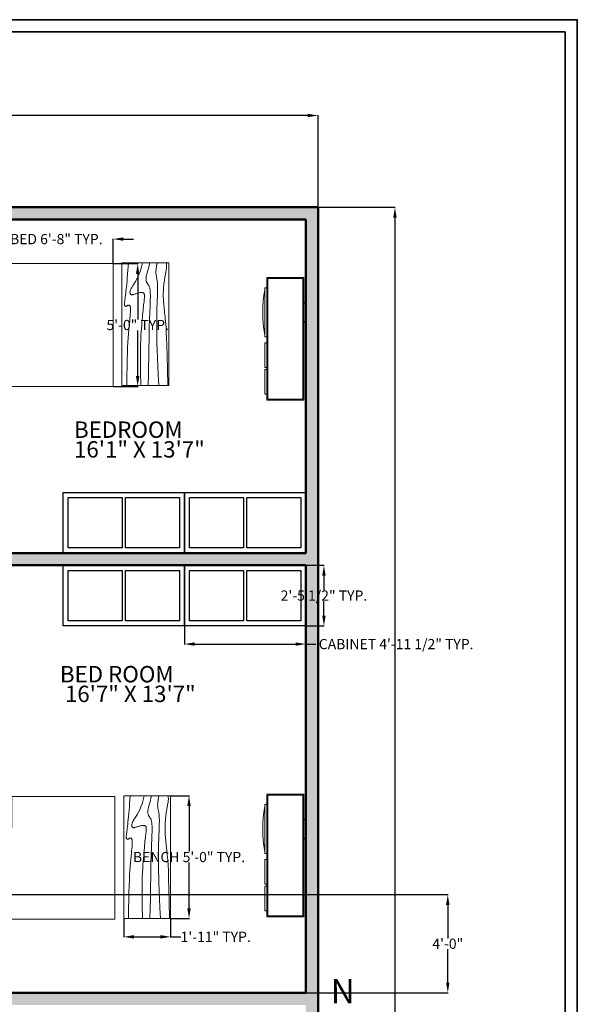
# Model space of a CAD drawing. Units: inches. Extents: x -60 to 743, y -483 to 510.
# Tile 7 of 7: x 470 to 743, y 29 to 510. Entities that reach past the tile are written whole.
import ezdxf

# ---------------------------------------------------------------- set-up
doc = ezdxf.new("R2010")
doc.units = ezdxf.units.IN
doc.header["$MEASUREMENT"] = 0
for name, color, linetype, lineweight in [('A-ANNO-DIMS', 2, 'Continuous', 18), ('A-ANNO-SYMB', 7, 'Continuous', 18), ('A-ANNO-TTLB', 7, 'Continuous', 35), ('A-AREA-IDEN', 7, 'Continuous', 25), ('A-FLOR-CASE', 40, 'Continuous', 25), ('A-WALL-PATT', 30, 'Continuous', 13), ('FURNITURE', 40, 'Continuous', 18), ('WALL BOUNDRY', 10, 'Continuous', 50)]:
    doc.layers.add(name, color=color, linetype=linetype, lineweight=lineweight)
doc.styles.get("Standard").update_dxf_attribs({"font": 'arial.ttf'})
doc.dimstyles.get("Standard").update_dxf_attribs({"dimtxt": 5, "dimasz": 5, "dimexe": 0.18, "dimexo": 0.0625, "dimgap": 0.09, "dimtad": 0, "dimtih": 1, "dimtoh": 1, "dimdec": 1, "dimzin": 0, "dimdsep": 46, "dimlunit": 4, "dimtxsty": 'Standard', "dimcen": 0.09, "dimadec": 0, "dimazin": 0, "dimtfac": 1, "dimtdec": 1, "dimtofl": 0, "dimtmove": 0, "dimatfit": 3, "dimfxl": 1, "dimtolj": 1, "dimtzin": 0, "dimarcsym": 0})

# ---------------------------------------------------------------- blocks, each defined once
blk = doc.blocks.new('Wall Cabinet - 18 x 36 in front')
for p, q in [((17.5, -1.5), (17.5, -16.5)), ((18.5, -16.5), (18.5, -1.5))]:
    blk.add_line(p, q)
blk.add_lwpolyline([(0, -18), (0, 0), (36, 0), (36, -18)], close=True)
for points in [[(17.5, -16.5), (1.5, -16.5), (1.5, -1.5), (17.5, -1.5)], [(18.5, -1.5), (34.5, -1.5), (34.5, -16.5), (18.5, -16.5)]]:
    blk.add_lwpolyline(points)
blk = doc.blocks.new('Bed - Queen')
for p, q in [((0, -80.00003), (0, 0)), ((0, 0), (59.99999, 0)), ((59.99999, 0), (59.99999, -80.00003)), ((7.99999, -1.2), (28.79998, -1.2)), ((7.99999, -14.4), (7.99999, -1.2)), ((28.79998, -1.2), (28.79998, -14.4)), ((31.19999, -1.2), (51.99999, -1.2)), ((31.19999, -14.4), (31.19999, -1.2)), ((51.99999, -1.2), (51.99999, -16.4)), ((0, -14.4), (44.8, -14.4)), ((59.99999, -29.6), (44.8, -14.4)), ((44.8, -14.4), (44.8, -29.6)), ((44.8, -16.8), (0, -16.8)), ((51.99999, -16.4), (46.79936, -16.4)), ((44.8, -29.6), (59.99999, -29.6)), ((59.99999, -80.00003), (0, -80.00003))]:
    blk.add_line(p, q)
blk = doc.blocks.new('Entertainment Center')
for p, q in [((-4, 0), (-5, -1)), ((4, 0), (-4, 0)), ((5, -1), (4, 0)), ((-17, -19), (-17, -1)), ((-17, -1), (43, -1)), ((-16.5, -18.5), (-16.5, -1.5)), ((-16.5, -1.5), (42.5, -1.5)), ((42.5, -1.5), (42.5, -18.5)), ((43, -1), (43, -19)), ((43, -19), (-17, -19)), ((42.5, -18.5), (-16.5, -18.5)), ((-12, -20), (-12, -19)), ((12, -19), (12, -20)), ((15, -20), (15, -19)), ((27, -19), (27, -20)), ((28, -20), (28, -19)), ((40, -19), (40, -20)), ((12, -20), (-12, -20)), ((27, -20), (15, -20)), ((40, -20), (28, -20))]:
    blk.add_line(p, q)
blk.add_arc((0, 40), 61, 259.6111, 280.3889)
blk = doc.blocks.new('*D22')
at = {"layer": 'A-ANNO-DIMS', "color": 0, "lineweight": -2, "transparency": 16777216}
for p, q in [((13.15, 418.48), (13.15, 463.48)), ((18.15, 463.3), (310.31, 463.3)), ((611.15, 463.3), (318.98, 463.3)), ((616.15, 418.48), (616.15, 463.48))]:
    blk.add_line(p, q, dxfattribs=at)
at = {"layer": 'A-ANNO-DIMS', "color": 0, "transparency": 16777216}
for points in [[(18.15, 464.13), (18.15, 462.46), (13.15, 463.3)], [(611.15, 464.13), (611.15, 462.46), (616.15, 463.3)]]:
    blk.add_solid(points, dxfattribs=at)
at = {"layer": 'Defpoints', "color": 0, "transparency": 16777216}
for p in [(616.15, 463.3), (13.15, 418.42), (616.15, 418.42)]:
    blk.add_point(p, dxfattribs=at)
at = {"layer": 'A-ANNO-DIMS', "color": 0, "transparency": 16777216, "insert": (314.65, 463.3), "char_height": 5, "attachment_point": 5}
blk.add_mtext("\\A1;50'", dxfattribs=at)
blk = doc.blocks.new('*D23')
at = {"layer": 'A-ANNO-DIMS', "color": 0, "lineweight": -2, "transparency": 16777216}
for p, q in [((616.21, 418.42), (653.91, 418.42)), ((653.73, 413.42), (653.73, 1.06)), ((653.73, -416.58), (653.73, -4.22)), ((616.21, -421.58), (653.91, -421.58))]:
    blk.add_line(p, q, dxfattribs=at)
at = {"layer": 'A-ANNO-DIMS', "color": 0, "transparency": 16777216}
for points in [[(652.9, 413.42), (654.56, 413.42), (653.73, 418.42)], [(652.9, -416.58), (654.56, -416.58), (653.73, -421.58)]]:
    blk.add_solid(points, dxfattribs=at)
at = {"layer": 'Defpoints', "color": 0, "transparency": 16777216}
for p in [(616.15, 418.42), (616.15, -421.58), (653.73, -421.58)]:
    blk.add_point(p, dxfattribs=at)
at = {"layer": 'A-ANNO-DIMS', "color": 0, "transparency": 16777216, "insert": (653.73, -1.58), "char_height": 5, "attachment_point": 5}
blk.add_mtext("\\A1;70'", dxfattribs=at)
blk = doc.blocks.new('BENCH-WOOD-60IN')
blk.add_lwpolyline([(22.9143, 0), (22.9143, 60), (0, 60), (0, 0)], close=True)
for points in [[(2.4, 0), (2.418, 4.8155), (2.4688, 9.0302), (2.5477, 12.709), (2.65, 15.9167), (2.7711, 18.7181), (2.9063, 21.1781), (3.0508, 23.3616), (3.2, 25.3333), (3.3495, 27.1477), (3.4958, 28.8172), (3.636, 30.3437), (3.7667, 31.7291), (3.8849, 32.9756), (3.9875, 34.0849), (4.0714, 35.059), (4.1334, 35.9), (4.1711, 36.6114), (4.1854, 37.2041), (4.1779, 37.6906), (4.15, 38.0833), (4.1034, 38.3948), (4.0396, 38.6375), (3.9602, 38.8239), (3.8667, 38.9666), (3.7608, 39.0764), (3.6448, 39.1573), (3.521, 39.2116), (3.3917, 39.2416), (3.2593, 39.2498), (3.1261, 39.2385), (2.9944, 39.21), (2.8667, 39.1666), (2.7447, 39.111), (2.6281, 39.0468), (2.5163, 38.978), (2.4083, 38.9083), (2.3035, 38.8418), (2.201, 38.7823), (2.1001, 38.7337), (2, 38.7), (1.9003, 38.6844), (1.8021, 38.6875), (1.707, 38.7094), (1.6167, 38.75), (1.5326, 38.8094), (1.4563, 38.8875), (1.3893, 38.9844), (1.3333, 39.1), (1.2896, 39.2351), (1.2583, 39.3937), (1.2396, 39.5804), (1.2333, 39.8), (1.2396, 40.057), (1.2583, 40.3562), (1.2896, 40.7023), (1.3333, 41.1), (1.3895, 41.5547), (1.4573, 42.0755), (1.5361, 42.6721), (1.625, 43.3542), (1.7233, 44.1316), (1.8302, 45.014), (1.9449, 46.0114), (2.0667, 47.1333), (2.1947, 48.3862), (2.3281, 49.7625), (2.4663, 51.2513), (2.6083, 52.8416), (2.7535, 54.5226), (2.9011, 56.2833), (3.0501, 58.1127), (3.2, 60)], [(9.2, 0), (9.0858, 6.5759), (9.0365, 11.9385), (9.0418, 16.2527), (9.0917, 19.6833), (9.1759, 22.3952), (9.2844, 24.5531), (9.4069, 26.322), (9.5333, 27.8666), (9.6553, 29.3241), (9.7719, 30.7203), (9.8837, 32.0532), (9.9917, 33.3208), (10.0965, 34.5213), (10.199, 35.6526), (10.2999, 36.7128), (10.4, 37.7), (10.4996, 38.6129), (10.5969, 39.4531), (10.6895, 40.223), (10.775, 40.925), (10.8512, 41.5613), (10.9156, 42.1344), (10.966, 42.6465), (11, 43.1), (11.0158, 43.4976), (11.0136, 43.8437), (10.9942, 44.143), (10.9583, 44.4), (10.9069, 44.6195), (10.8406, 44.8062), (10.7603, 44.9648), (10.6667, 45.1), (10.5598, 45.2155), (10.4365, 45.3114), (10.2929, 45.3871), (10.125, 45.4416), (9.929, 45.4743), (9.7011, 45.4844), (9.4371, 45.4709), (9.1333, 45.4333), (8.7883, 45.3716), (8.4104, 45.2896), (8.0107, 45.1919), (7.6, 45.0833), (7.1893, 44.9685), (6.7896, 44.8521), (6.4117, 44.7388), (6.0667, 44.6333), (5.7628, 44.54), (5.4979, 44.4614), (5.2675, 44.4001), (5.0667, 44.3583), (4.8909, 44.3384), (4.7354, 44.3427), (4.5956, 44.3736), (4.4667, 44.4333), (4.3453, 44.5236), (4.2333, 44.6427), (4.1339, 44.7884), (4.05, 44.9583), (3.9849, 45.1501), (3.9417, 45.3614), (3.9234, 45.59), (3.9333, 45.8333), (3.9749, 46.0915), (4.0531, 46.3734), (4.1736, 46.6906), (4.3417, 47.0542), (4.5629, 47.4756), (4.8427, 47.9661), (5.1866, 48.5372), (5.6, 49.2), (6.0844, 49.9676), (6.625, 50.8594), (7.2031, 51.8965), (7.8, 53.1), (8.3969, 54.491), (8.975, 56.0906), (9.5156, 57.9199), (10, 60)], [(12.8, 0), (12.9322, 5.1847), (13.0323, 9.6213), (13.1059, 13.3963), (13.1583, 16.5958), (13.1952, 19.3063), (13.2219, 21.614), (13.2439, 23.6054), (13.2667, 25.3666), (13.2947, 26.9728), (13.3281, 28.4531), (13.3663, 29.8256), (13.4083, 31.1083), (13.4535, 32.3191), (13.501, 33.476), (13.5501, 34.597), (13.6, 35.7), (13.6497, 36.7984), (13.6979, 37.8875), (13.743, 38.9578), (13.7833, 40), (13.8174, 41.0047), (13.8438, 41.9625), (13.8607, 42.864), (13.8667, 43.7), (13.8604, 44.4631), (13.8417, 45.1552), (13.8104, 45.7801), (13.7667, 46.3416), (13.7104, 46.8439), (13.6417, 47.2906), (13.5604, 47.6858), (13.4667, 48.0333), (13.3608, 48.3375), (13.2448, 48.6042), (13.121, 48.8396), (12.9917, 49.05), (12.8593, 49.2417), (12.7261, 49.4208), (12.5944, 49.5937), (12.4667, 49.7667), (12.3451, 49.9452), (12.2313, 50.1323), (12.1268, 50.3303), (12.0333, 50.5416), (11.9524, 50.7686), (11.8854, 51.0135), (11.8341, 51.2788), (11.8, 51.5666), (11.7843, 51.8785), (11.7865, 52.2116), (11.8059, 52.562), (11.8417, 52.926), (11.8931, 53.2998), (11.9594, 53.6795), (12.0397, 54.0614), (12.1333, 54.4416), (12.2401, 54.8223), (12.3625, 55.2293), (12.5037, 55.6942), (12.6667, 56.2489), (12.8547, 56.9251), (13.0708, 57.7545), (13.3182, 58.7689), (13.6, 60)], [(18, 0), (17.7273, 5.124), (17.5057, 9.6609), (17.3303, 13.6705), (17.1958, 17.2125), (17.0973, 20.3467), (17.0297, 23.1328), (16.9878, 25.6307), (16.9667, 27.9), (16.9617, 29.9928), (16.9703, 31.9302), (16.9907, 33.7254), (17.0208, 35.3917), (17.0588, 36.9423), (17.1026, 38.3906), (17.1503, 39.7499), (17.2, 41.0333), (17.2496, 42.2519), (17.2969, 43.4073), (17.3395, 44.4986), (17.375, 45.525), (17.4012, 46.4858), (17.4156, 47.3802), (17.416, 48.2074), (17.4, 48.9667), (17.3662, 49.6583), (17.3167, 50.2872), (17.2547, 50.8595), (17.1833, 51.3812), (17.1057, 51.8584), (17.025, 52.2971), (16.9443, 52.7034), (16.8667, 53.0833), (16.7951, 53.443), (16.7313, 53.789), (16.6768, 54.128), (16.6334, 54.4666), (16.6024, 54.8115), (16.5854, 55.1693), (16.5841, 55.5465), (16.6, 55.95), (16.6337, 56.3828), (16.6823, 56.8346), (16.7418, 57.2915), (16.8084, 57.7396), (16.878, 58.165), (16.9469, 58.5539), (17.0111, 58.8924), (17.0667, 59.1666), (17.1107, 59.3679), (17.1438, 59.5078), (17.1675, 59.6032), (17.1833, 59.6708), (17.193, 59.7275), (17.1979, 59.7901), (17.1998, 59.8753), (17.2, 60)], [(22.4, 0), (22.2501, 8.0098), (22.1011, 14.4094), (21.9535, 19.4168), (21.8083, 23.25), (21.6663, 26.1269), (21.5281, 28.2656), (21.3947, 29.884), (21.2667, 31.2), (21.1448, 32.3967), (21.0292, 33.5172), (20.9198, 34.5697), (20.8167, 35.5625), (20.7198, 36.5037), (20.6292, 37.4015), (20.5448, 38.2642), (20.4667, 39.1), (20.3951, 39.9164), (20.3313, 40.7187), (20.2768, 41.5117), (20.2333, 42.3), (20.2024, 43.0883), (20.1854, 43.8812), (20.1841, 44.6836), (20.2, 45.5), (20.234, 46.3328), (20.2844, 47.1747), (20.3488, 48.0163), (20.425, 48.8479), (20.5106, 49.66), (20.6031, 50.4429), (20.7004, 51.1872), (20.8, 51.8833), (20.8999, 52.5246), (20.9995, 53.1166), (21.0983, 53.6681), (21.1958, 54.1875), (21.2919, 54.6834), (21.3859, 55.1646), (21.4777, 55.6394), (21.5667, 56.1167), (21.6515, 56.6028), (21.7266, 57.0961), (21.7852, 57.5929), (21.8208, 58.0896), (21.8268, 58.5823), (21.7964, 59.0674), (21.723, 59.5412), (21.6, 60)]]:
    blk.add_lwpolyline(points)
blk = doc.blocks.new('*D30')
at = {"layer": 'A-ANNO-DIMS', "color": 0, "lineweight": -2, "transparency": 16777216}
for p, q in [((550.88, 213.73), (550.88, 204.72)), ((610.15, 213.73), (610.15, 204.72)), ((555.88, 204.9), (605.15, 204.9)), ((610.15, 204.9), (615.15, 204.9))]:
    blk.add_line(p, q, dxfattribs=at)
at = {"layer": 'A-ANNO-DIMS', "color": 0, "transparency": 16777216}
for points in [[(555.88, 205.73), (555.88, 204.07), (550.88, 204.9)], [(605.15, 205.73), (605.15, 204.07), (610.15, 204.9)]]:
    blk.add_solid(points, dxfattribs=at)
at = {"layer": 'Defpoints', "color": 0, "transparency": 16777216}
for p in [(550.88, 213.79), (610.15, 213.79), (610.15, 204.9)]:
    blk.add_point(p, dxfattribs=at)
at = {"layer": 'A-ANNO-DIMS', "color": 0, "transparency": 16777216, "insert": (654.32, 204.9), "char_height": 5, "attachment_point": 5}
blk.add_mtext('\\A1;CABINET 4\'-11 1/2" TYP.', dxfattribs=at)
blk = doc.blocks.new('*D31')
at = {"layer": 'A-ANNO-DIMS', "color": 0, "lineweight": -2, "transparency": 16777216}
for p, q in [((610.21, 243.42), (619.22, 243.42)), ((619.04, 238.42), (619.04, 231.28)), ((619.04, 218.79), (619.04, 225.93)), ((610.21, 213.79), (619.22, 213.79))]:
    blk.add_line(p, q, dxfattribs=at)
at = {"layer": 'A-ANNO-DIMS', "color": 0, "transparency": 16777216}
for points in [[(618.2, 238.42), (619.87, 238.42), (619.04, 243.42)], [(618.2, 218.79), (619.87, 218.79), (619.04, 213.79)]]:
    blk.add_solid(points, dxfattribs=at)
at = {"layer": 'Defpoints', "color": 0, "transparency": 16777216}
for p in [(610.15, 243.42), (619.04, 243.42), (610.15, 213.79)]:
    blk.add_point(p, dxfattribs=at)
at = {"layer": 'A-ANNO-DIMS', "color": 0, "transparency": 16777216, "insert": (619.04, 228.61), "char_height": 5, "attachment_point": 5}
blk.add_mtext('\\A1;2\'-5 1/2" TYP.', dxfattribs=at)
blk = doc.blocks.new('*D50')
at = {"layer": 'A-ANNO-DIMS', "color": 0, "lineweight": -2, "transparency": 16777216}
for p, q in [((431.03, 402.88), (426.03, 402.88)), ((436.03, 390.95), (436.03, 403.06)), ((516.03, 390.95), (516.03, 403.06)), ((521.03, 402.88), (526.03, 402.88))]:
    blk.add_line(p, q, dxfattribs=at)
at = {"layer": 'A-ANNO-DIMS', "color": 0, "transparency": 16777216}
for points in [[(431.03, 403.72), (431.03, 402.05), (436.03, 402.88)], [(521.03, 403.72), (521.03, 402.05), (516.03, 402.88)]]:
    blk.add_solid(points, dxfattribs=at)
at = {"layer": 'Defpoints', "color": 0, "transparency": 16777216}
for p in [(436.03, 402.88), (436.03, 390.88), (516.03, 390.88)]:
    blk.add_point(p, dxfattribs=at)
at = {"layer": 'A-ANNO-DIMS', "color": 0, "transparency": 16777216, "insert": (476.03, 402.88), "char_height": 5, "attachment_point": 5}
blk.add_mtext('\\A1;QUEEN BED 6\'-8" TYP.', dxfattribs=at)
blk = doc.blocks.new('*D51')
at = {"layer": 'A-ANNO-DIMS', "color": 0, "lineweight": -2, "transparency": 16777216}
for p, q in [((516.09, 390.88), (528.21, 390.88)), ((528.03, 385.88), (528.03, 363.53)), ((528.03, 335.88), (528.03, 358.24)), ((516.09, 330.88), (528.21, 330.88))]:
    blk.add_line(p, q, dxfattribs=at)
at = {"layer": 'A-ANNO-DIMS', "color": 0, "transparency": 16777216}
for points in [[(527.19, 385.88), (528.86, 385.88), (528.03, 390.88)], [(527.19, 335.88), (528.86, 335.88), (528.03, 330.88)]]:
    blk.add_solid(points, dxfattribs=at)
at = {"layer": 'Defpoints', "color": 0, "transparency": 16777216}
for p in [(516.03, 390.88), (528.03, 390.88), (516.03, 330.88)]:
    blk.add_point(p, dxfattribs=at)
at = {"layer": 'A-ANNO-DIMS', "color": 0, "transparency": 16777216, "insert": (528.03, 360.88), "char_height": 5, "attachment_point": 5}
blk.add_mtext('\\A1;5\'-0" TYP.', dxfattribs=at)
blk = doc.blocks.new('*D52')
at = {"layer": 'A-ANNO-DIMS', "color": 0, "lineweight": -2, "transparency": 16777216}
for p, q in [((544.18, 130.8), (553.29, 130.8)), ((553.11, 125.8), (553.11, 103.47)), ((553.11, 75.8), (553.11, 98.12)), ((544.18, 70.8), (553.29, 70.8))]:
    blk.add_line(p, q, dxfattribs=at)
at = {"layer": 'A-ANNO-DIMS', "color": 0, "transparency": 16777216}
for points in [[(552.28, 125.8), (553.95, 125.8), (553.11, 130.8)], [(552.28, 75.8), (553.95, 75.8), (553.11, 70.8)]]:
    blk.add_solid(points, dxfattribs=at)
at = {"layer": 'Defpoints', "color": 0, "transparency": 16777216}
for p in [(544.11, 130.8), (553.11, 130.8), (544.11, 70.8)]:
    blk.add_point(p, dxfattribs=at)
at = {"layer": 'A-ANNO-DIMS', "color": 0, "transparency": 16777216, "insert": (553.11, 100.8), "char_height": 5, "attachment_point": 5}
blk.add_mtext('\\A1;BENCH 5\'-0" TYP.', dxfattribs=at)
blk = doc.blocks.new('*D53')
at = {"layer": 'A-ANNO-DIMS', "color": 0, "lineweight": -2, "transparency": 16777216}
for p, q in [((521.2, 70.74), (521.2, 61.62)), ((544.11, 70.74), (544.11, 61.62)), ((526.2, 61.8), (539.11, 61.8)), ((544.11, 61.8), (549.11, 61.8))]:
    blk.add_line(p, q, dxfattribs=at)
at = {"layer": 'A-ANNO-DIMS', "color": 0, "transparency": 16777216}
for points in [[(526.2, 62.63), (526.2, 60.97), (521.2, 61.8)], [(539.11, 62.63), (539.11, 60.97), (544.11, 61.8)]]:
    blk.add_solid(points, dxfattribs=at)
at = {"layer": 'Defpoints', "color": 0, "transparency": 16777216}
for p in [(521.2, 70.8), (544.11, 70.8), (544.11, 61.8)]:
    blk.add_point(p, dxfattribs=at)
at = {"layer": 'A-ANNO-DIMS', "color": 0, "transparency": 16777216, "insert": (566.15, 61.8), "char_height": 5, "attachment_point": 5}
blk.add_mtext('\\A1;1\'-11" TYP.', dxfattribs=at)
blk = doc.blocks.new('*D74')
at = {"layer": 'A-ANNO-DIMS', "color": 0, "lineweight": -2, "transparency": 16777216}
for p, q in [((187.21, 82.42), (679.73, 82.42)), ((679.55, 77.42), (679.55, 61.06)), ((679.55, 39.42), (679.55, 55.78)), ((187.21, 34.42), (679.73, 34.42))]:
    blk.add_line(p, q, dxfattribs=at)
at = {"layer": 'A-ANNO-DIMS', "color": 0, "transparency": 16777216}
for points in [[(678.72, 77.42), (680.39, 77.42), (679.55, 82.42)], [(678.72, 39.42), (680.39, 39.42), (679.55, 34.42)]]:
    blk.add_solid(points, dxfattribs=at)
at = {"layer": 'Defpoints', "color": 0, "transparency": 16777216}
for p in [(187.15, 82.42), (679.55, 82.42), (187.15, 34.42)]:
    blk.add_point(p, dxfattribs=at)
at = {"layer": 'A-ANNO-DIMS', "color": 0, "transparency": 16777216, "insert": (679.55, 58.42), "char_height": 5, "attachment_point": 5}
blk.add_mtext('\\A1;4\'-0"', dxfattribs=at)

msp = doc.modelspace()

# ---------------------------------------------------------------- hatches: boundary and pattern name
at = {"layer": 'A-WALL-PATT'}
h = msp.add_hatch(color=256, dxfattribs=at)
h.dxf.hatch_style = 1
h.paths.add_polyline_path([(412.35, 168.77), (415.89, 168.77), (415.89, 114.92), (412.35, 114.92)], flags=16)
h.paths.add_polyline_path([(87.81, -138.81), (87.81, -142.35), (48.31, -142.32), (48.31, -138.78)], flags=16)
h.paths.add_polyline_path([(459.53, -138.78), (513.39, -138.78), (513.39, -142.32), (459.53, -142.32)], flags=16)
h.paths.add_polyline_path([(164.84, -257.78), (218.7, -257.78), (218.7, -261.32), (164.84, -261.32)], flags=16)
h.paths.add_polyline_path([(417.15, 114.92), (415.89, 114.92), (415.89, 168.77), (417.15, 168.77), (417.15, 195.42), (411.15, 195.42), (411.15, 168.77), (412.35, 168.77), (412.35, 114.92), (411.15, 114.92), (411.15, 28.42), (610.15, 28.42), (610.15, -43.58), (508.15, -43.58), (508.15, -49.58), (610.15, -49.58), (610.15, -137.58), (513.39, -137.58), (513.39, -138.78), (459.53, -138.78), (459.53, -137.58), (359.15, -137.58), (359.15, -143.58), (377.15, -143.58), (377.15, -292.58), (383.15, -292.58), (383.15, -143.58), (459.53, -143.58), (459.53, -142.32), (513.39, -142.32), (513.39, -143.58), (610.15, -143.58), (610.15, -415.58), (610.15, -421.58), (616.15, -421.58), (616.15, 418.42), (13.15, 418.42), (13.15, -421.58), (19.15, -421.58), (430.15, -421.58), (430.15, -415.58), (19.15, -415.58), (19.15, -143.58), (48.31, -143.58), (48.31, -142.32), (87.81, -142.35), (87.81, -143.58), (117.15, -143.58), (117.15, -262.58), (164.84, -262.58), (164.84, -261.32), (218.7, -261.32), (218.7, -262.58), (273.15, -262.58), (273.15, -292.58), (279.15, -292.58), (279.15, -143.58), (297.15, -143.58), (297.15, -137.58), (273.15, -137.58), (273.15, -256.58), (218.7, -256.58), (218.7, -257.78), (164.84, -257.78), (164.84, -256.58), (123.15, -256.58), (123.15, -143.58), (225.15, -143.58), (225.15, -137.58), (87.81, -137.58), (87.81, -138.81), (48.31, -138.78), (48.31, -137.58), (19.15, -137.58), (19.15, 28.42), (187.15, 28.42), (187.15, 34.42), (19.15, 34.42), (19.15, 178.42), (273.15, 178.42), (273.15, 184.42), (19.15, 184.42), (19.15, 345.58), (195.14, 345.58), (195.14, 348.9), (19.15, 348.9), (19.15, 412.42), (267.15, 412.42), (267.15, 319.83), (273.15, 319.83), (273.15, 412.42), (411.15, 412.42), (411.15, 376.24), (417.15, 376.24), (417.15, 412.42), (610.15, 412.42), (610.15, 249.42), (411.15, 249.42), (411.15, 243.42), (610.15, 243.42), (610.15, 34.42), (417.15, 34.42)])

# ---------------------------------------------------------------- linework, layer by layer
at = {"layer": 'A-ANNO-TTLB'}
for points in [[(742.84, -483.31), (-60.19, -483.31), (-60.19, 510.12), (742.84, 510.12)], [(736.84, -477.31), (-54.19, -477.31), (-54.19, 504.12), (736.84, 504.12)]]:
    msp.add_lwpolyline(points, close=True, dxfattribs=at)
at = {"layer": 'WALL BOUNDRY'}
msp.add_lwpolyline([(610.15, -415.58), (610.15, -421.58), (616.15, -421.58), (616.15, 418.42), (13.15, 418.42), (13.15, -421.58), (19.15, -421.58), (430.15, -421.58), (430.15, -415.58), (19.15, -415.58), (19.15, -143.58), (117.15, -143.58), (117.15, -262.58), (273.15, -262.58), (273.15, -292.58), (279.15, -292.58), (377.15, -292.58), (383.15, -292.58), (383.15, -143.58), (610.15, -143.58)], close=True, dxfattribs=at)
for points in [[(417.15, 412.42), (610.15, 412.42), (610.15, 249.42), (411.15, 249.42)], [(411.15, 243.42), (610.15, 243.42), (610.15, 34.42), (417.15, 34.42)]]:
    msp.add_lwpolyline(points, dxfattribs=at)

# ---------------------------------------------------------------- block references
at = {"layer": 'A-FLOR-CASE', "xscale": 1.646250125450342, "yscale": 1.646250125450342, "zscale": 1.646250125450342}
for p in [(491.62, 279.05), (550.88, 279.05), (491.62, 243.42), (550.88, 243.42)]:
    msp.add_blockref('Wall Cabinet - 18 x 36 in front', p, dxfattribs=at)
at = {"layer": 'FURNITURE'}
for name, p, rotation in [('Bed - Queen', (436.03, 330.88), 90), ('Entertainment Center', (610.15, 367.12), 270), ('Bed - Queen', (436.88, 70.36), 90), ('Entertainment Center', (610.15, 114.53), 270)]:
    msp.add_blockref(name, p, dxfattribs=dict(at, rotation=rotation))
for p in [(520.35, 331.32), (521.2, 70.8)]:
    msp.add_blockref('BENCH-WOOD-60IN', p, dxfattribs=at)

# ---------------------------------------------------------------- texts
at = {"layer": 'A-ANNO-SYMB'}
msp.add_text('N', height=12, dxfattribs=at).set_placement((622.31, 29.21))
at = {"layer": 'A-AREA-IDEN'}
for s, p in [('BEDROOM', (496.91, 305.72)), ('16\'1" X 13\'7"', (496.91, 296.08)), ('BED ROOM ', (490.02, 186.19)), (' 16\'7" X 13\'7"', (490.02, 176.56))]:
    msp.add_text(s, height=8, dxfattribs=at).set_placement(p)

# ---------------------------------------------------------------- dimensions: what is measured, and where the dimension line sits
at = {"layer": 'A-ANNO-DIMS'}
for base, p1, p2, text, override, picture, middle in [((616.15, 463.3), (13.15, 418.42), (616.15, 418.42), "50'", {"dimclrd": 0, "dimclre": 0, "dimclrt": 0}, '*D22', (314.65, 463.3)), ((610.15, 204.9), (550.88, 213.79), (610.15, 213.79), 'CABINET <> TYP.', {"dimdec": 1, "dimlfac": 1, "dimrnd": 0, "dimzin": 1, "dimdsep": 46, "dimlunit": 4, "dimfrac": 2}, '*D30', (654.32, 204.9)), ((544.11, 61.8), (521.2, 70.8), (544.11, 70.8), '<> TYP.', {"dimdec": 1, "dimlfac": 1, "dimrnd": 0, "dimzin": 1, "dimdsep": 46, "dimlunit": 4, "dimfrac": 2}, '*D53', (566.15, 61.8))]:
    dim = msp.add_linear_dim(base=base, p1=p1, p2=p2, text=text, dimstyle='Standard', override=override, dxfattribs=at)
    dim.commit()
    dim.dimension.update_dxf_attribs({"geometry": picture, "text_midpoint": middle})
for base, p1, p2, angle, text, picture, middle in [((436.03, 402.88), (516.03, 390.88), (436.03, 390.88), 180, 'QUEEN BED <> TYP.', '*D50', (476.03, 402.88)), ((528.03, 390.88), (516.03, 330.88), (516.03, 390.88), 90, '<> TYP.', '*D51', (528.03, 360.88)), ((619.04, 243.42), (610.15, 213.79), (610.15, 243.42), 90, '<> TYP.', '*D31', (619.04, 228.61)), ((553.11, 130.8), (544.11, 70.8), (544.11, 130.8), 90, 'BENCH <> TYP.', '*D52', (553.11, 100.8))]:
    dim = msp.add_linear_dim(base=base, p1=p1, p2=p2, angle=angle, text=text, dimstyle='Standard', override={"dimdec": 1, "dimlfac": 1, "dimrnd": 0, "dimzin": 1, "dimdsep": 46, "dimlunit": 4, "dimfrac": 2}, dxfattribs=at)
    dim.commit()
    dim.dimension.update_dxf_attribs({"geometry": picture, "text_midpoint": middle})
for base, p1, p2, override, picture, middle in [((653.73, -421.58), (616.15, 418.42), (616.15, -421.58), {"dimclrd": 0, "dimclre": 0, "dimclrt": 0}, '*D23', (653.73, -1.58)), ((679.55, 82.42), (187.15, 34.42), (187.15, 82.42), {"dimdec": 1, "dimlfac": 1, "dimrnd": 0, "dimzin": 1, "dimdsep": 46, "dimlunit": 4, "dimfrac": 2}, '*D74', (679.55, 58.42))]:
    dim = msp.add_linear_dim(base=base, p1=p1, p2=p2, angle=90, dimstyle='Standard', override=override, dxfattribs=at)
    dim.commit()
    dim.dimension.update_dxf_attribs({"geometry": picture, "text_midpoint": middle})

doc.saveas('drawing.dxf')
